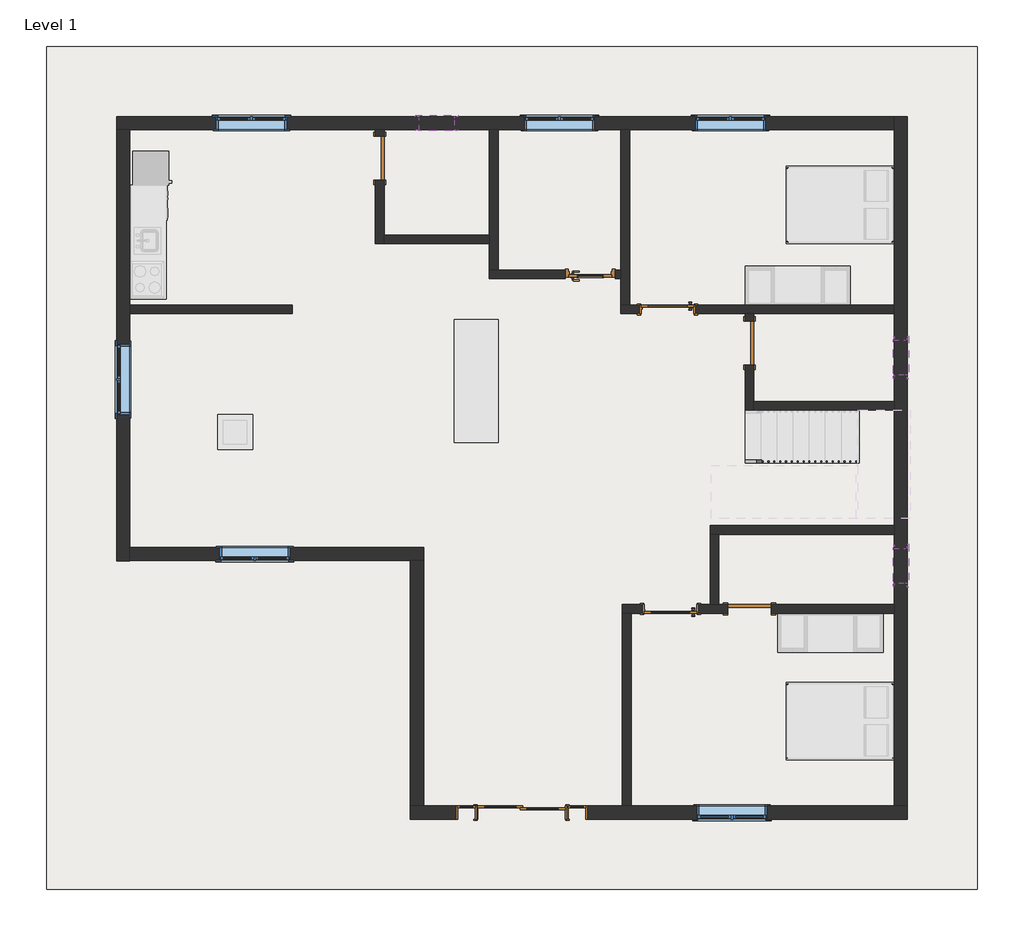
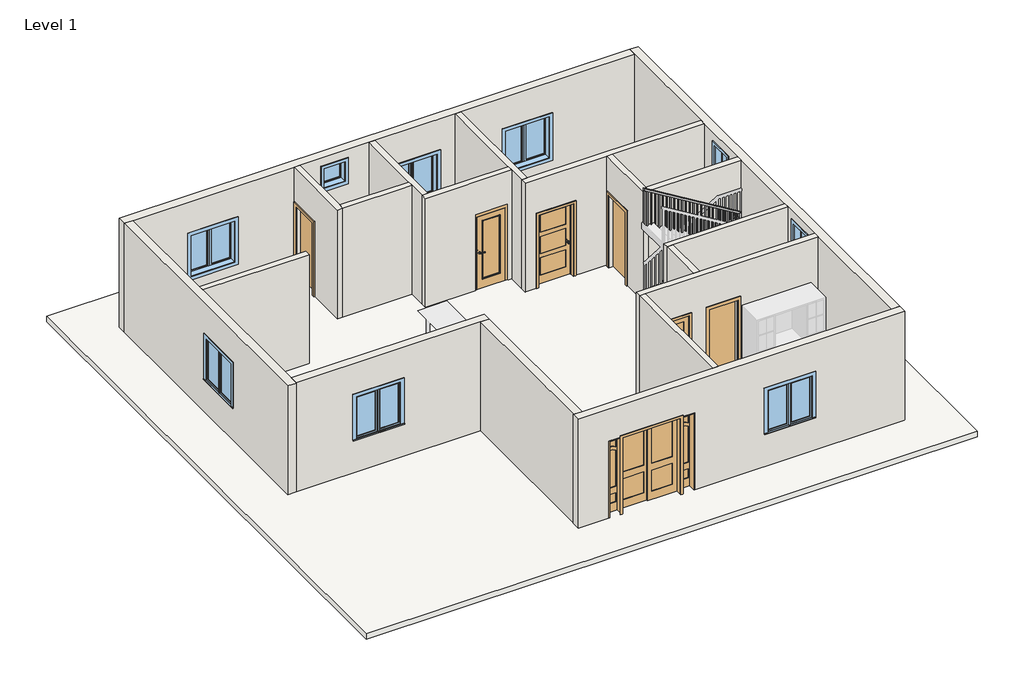
# One storey, part 1 of 2: 19 walls, 9 doors, 9 windows, 1 railing, 1 slab.
"""IFC4 building model written with IfcOpenShell, lengths in millimetres."""

from ifc_helpers import new_model, si_unit, frame, origin, origin_with_axes, place, context, project, spatial, polyline, outline, extrude, faceted_brep, transform, mapped, element, save
from components import door_0052078e, door_302e125b, door_f5864cb8, door_ac27962c, door_c5233792, door_136239c3, door_d64d7266, window_534dcd48, window_3ed046d9

model = new_model("IFC4")

# Units and contexts
model_context = context("Model", 3, world=origin())
ifc_project = project(units=[si_unit("LENGTHUNIT", "METRE", prefix="MILLI")], contexts=[model_context])

# Site, building, storey
site = spatial("IfcSite", under=ifc_project)
building = spatial("IfcBuilding", under=site)
storey = spatial("IfcBuildingStorey", under=building, Name="Level 1", Elevation=0.0)

# Doors
placement = place(None, origin())
door_shape = door_0052078e(model_context)
element("IfcDoor", 1, ObjectType="12\" x 84\"", at=placement, inside=storey, context=model_context, shape_type="MappedRepresentation", body=[
    mapped(door_shape, transform((-8475.4866603, -9530.4581121, 0.0), x_axis=(1.0, 0.0, 0.0), y_axis=(0.0, 1.0, 0.0), z_axis=(0.0, 0.0, 1.0))),
])
door_2_shape = door_302e125b(model_context)
element("IfcDoor", 2, ObjectType="12\" x 84\"", at=placement, inside=storey, context=model_context, shape_type="MappedRepresentation", body=[
    mapped(door_2_shape, transform((-6557.7866603, -9530.4581121, 0.0), x_axis=(-1.0, 0.0, 0.0), y_axis=(0.0, -1.0, 0.0), z_axis=(0.0, 0.0, 1.0))),
])
door_3_shape = door_f5864cb8(model_context)
element("IfcDoor", 3, ObjectType="Door-Interior-Double-Sliding-2_Panel-Wood : 60\" x 84\"", at=placement, inside=storey, context=model_context, shape_type="MappedRepresentation", body=[
    mapped(door_3_shape, transform((-7522.9866603, -9530.4581121, 0.0), x_axis=(1.0, 0.0, 0.0), y_axis=(0.0, 1.0, 0.0), z_axis=(0.0, 0.0, 1.0))),
])
door_4_shape = door_ac27962c(model_context)
element("IfcDoor", 4, ObjectType="Door-Interior-Single-3_Panel_Vert-Wood : 36\" x 80\"", at=placement, inside=storey, context=model_context, shape_type="MappedRepresentation", body=[
    mapped(door_4_shape, transform((-4932.1866603, -5993.5081121, 0.0), x_axis=(-1.0, 0.0, 0.0), y_axis=(0.0, -1.0, 0.0), z_axis=(0.0, 0.0, 1.0))),
])
door_5_shape = door_c5233792(model_context)
element("IfcDoor", 5, ObjectType="Door-Interior-Single-3_Panel_Vert-Wood : 36\" x 80\"", at=placement, inside=storey, context=model_context, shape_type="MappedRepresentation", body=[
    mapped(door_5_shape, transform((-4982.9866603, -780.1581121, 0.0), x_axis=(-1.0, 0.0, 0.0), y_axis=(0.0, -1.0, 0.0), z_axis=(0.0, 0.0, 1.0))),
])
door_6_shape = door_136239c3(model_context)
element("IfcDoor", 6, ObjectType="Door-Passage-Single-Full_Lite : 30\" x 80\"", at=placement, inside=storey, context=model_context, shape_type="MappedRepresentation", body=[
    mapped(door_6_shape, transform((-6329.1866603, -167.3831121, 0.0), x_axis=(1.0, 0.0, 0.0), y_axis=(0.0, 1.0, 0.0), z_axis=(0.0, 0.0, 1.0))),
])
door_7_shape = door_d64d7266(model_context)
element("IfcDoor", 7, ObjectType="Door-Single-Panel : 30\" x 80\"", at=placement, inside=storey, context=model_context, shape_type="MappedRepresentation", body=[
    mapped(door_7_shape, transform((-3560.5866603, -5990.3331121, 0.0), x_axis=(-1.0, 0.0, 0.0), y_axis=(0.0, -1.0, 0.0), z_axis=(0.0, 0.0, 1.0))),
])
element("IfcDoor", 8, ObjectType="Door-Single-Panel : 30\" x 80\"", at=placement, inside=storey, context=model_context, shape_type="MappedRepresentation", body=[
    mapped(door_7_shape, transform((-3560.5866603, -1367.5331121, 0.0), x_axis=(0.0, 1.0, 0.0), y_axis=(-1.0, 0.0, 0.0), z_axis=(0.0, 0.0, 1.0))),
])
element("IfcDoor", 9, ObjectType="Door-Single-Panel : 30\" x 80\"", at=placement, inside=storey, context=model_context, shape_type="MappedRepresentation", body=[
    mapped(door_7_shape, transform((-9986.7866603, 1845.5668879, 0.0), x_axis=(0.0, 1.0, 0.0), y_axis=(-1.0, 0.0, 0.0), z_axis=(0.0, 0.0, 1.0))),
])

# Railing
element("IfcRailing", 10, ObjectType="Handrail - Rectangular", at=placement, inside=storey, context=model_context, shape_type="SolidModel", body=[
    faceted_brep([(-3636.7866603, -3399.5331121, 1083.7333333), (-3636.7866603, -3399.5331121, 1024.3318731), (-3636.7866603, -3450.3331121, 1024.3318731), (-3636.7866603, -3450.3331121, 1083.7333333), (-1757.1866603, -3399.5331121, 2222.8848485), (-1706.3866603, -3399.5331121, 2194.271267), (-1706.3866603, -3450.3331121, 2194.271267), (-1757.1866603, -3450.3331121, 2222.8848485), (-1757.1866603, -3399.5331121, 2269.0666667), (-1706.3866603, -3399.5331121, 2218.2666667), (-1706.3866603, -3450.3331121, 2218.2666667), (-1757.1866603, -3450.3331121, 2269.0666667), (-1630.1866603, -3399.5331121, 2269.0666667), (-1630.1866603, -3399.5331121, 2218.2666667), (-1680.9866603, -3450.3331121, 2218.2666667), (-1680.9866603, -3450.3331121, 2269.0666667), (-1630.1866603, -3501.1331121, 2269.0666667), (-1680.9866603, -3501.1331121, 2269.0666667), (-1680.9866603, -3551.9331121, 2218.2666667), (-1630.1866603, -3551.9331121, 2218.2666667)], [[[0, 1, 2, 3]], [[1, 0, 4, 5]], [[2, 1, 5, 6]], [[3, 2, 6, 7]], [[0, 3, 7, 4]], [[5, 4, 8, 9]], [[6, 5, 9, 10]], [[7, 6, 10, 11]], [[4, 7, 11, 8]], [[9, 8, 12, 13]], [[10, 9, 13, 14]], [[11, 10, 14, 15]], [[8, 11, 15, 12]], [[16, 17, 18, 19]], [[13, 12, 16, 19]], [[14, 13, 19, 18]], [[15, 14, 18, 17]], [[12, 15, 17, 16]]]),
    faceted_brep([(-1630.1866603, -3501.1331121, 2269.0666667), (-1630.1866603, -3551.9331121, 2218.2666667), (-1680.9866603, -3551.9331121, 2218.2666667), (-1680.9866603, -3501.1331121, 2269.0666667), (-1630.1866603, -3501.1331121, 2407.6121212), (-1680.9866603, -3501.1331121, 2378.9985397), (-1680.9866603, -3551.9331121, 2378.9985397), (-1630.1866603, -3551.9331121, 2407.6121212)], [[[0, 1, 2, 3]], [[4, 5, 6, 7]], [[1, 0, 4, 7]], [[2, 1, 7, 6]], [[3, 2, 6, 5]], [[0, 3, 5, 4]]]),
    faceted_brep([(-1630.1866603, -3551.9331121, 2407.6121212), (-1680.9866603, -3551.9331121, 2378.9985397), (-1680.9866603, -3501.1331121, 2378.9985397), (-1630.1866603, -3501.1331121, 2407.6121212), (-4195.5866603, -3551.9331121, 3962.4), (-4195.5866603, -3501.1331121, 3962.4), (-4195.5866603, -3501.1331121, 3902.9985397), (-4195.5866603, -3551.9331121, 3902.9985397)], [[[0, 1, 2, 3]], [[4, 5, 6, 7]], [[1, 0, 4, 7]], [[2, 1, 7, 6]], [[3, 2, 6, 5]], [[0, 3, 5, 4]]]),
    extrude(outline(polyline([(3835.6500549, -4084.4616603), (3847.1955094, -4103.5116603), (2878.6666667, -4103.5116603), (2878.6666667, -4084.4616603), (3835.6500549, -4084.4616603)])), frame((0.0, -3536.0581121, 0.0), z_axis=(0.0, 1.0, 0.0), x_axis=(0.0, 0.0, 1.0)), (0.0, 0.0, 1.0), 19.05),
    extrude(outline(polyline([(3774.0742973, -3982.8616603), (3785.6197519, -4001.9116603), (2878.6666667, -4001.9116603), (2878.6666667, -3982.8616603), (3774.0742973, -3982.8616603)])), frame((0.0, -3536.0581121, 0.0), z_axis=(0.0, 1.0, 0.0), x_axis=(0.0, 0.0, 1.0)), (0.0, 0.0, 1.0), 19.05),
    extrude(outline(polyline([(3712.4985397, -3881.2616603), (3724.0439943, -3900.3116603), (2709.3333333, -3900.3116603), (2709.3333333, -3881.2616603), (3712.4985397, -3881.2616603)])), frame((0.0, -3536.0581121, 0.0), z_axis=(0.0, 1.0, 0.0), x_axis=(0.0, 0.0, 1.0)), (0.0, 0.0, 1.0), 19.05),
    extrude(outline(polyline([(3650.9227822, -3779.6616603), (3662.4682367, -3798.7116603), (2709.3333333, -3798.7116603), (2709.3333333, -3779.6616603), (3650.9227822, -3779.6616603)])), frame((0.0, -3536.0581121, 0.0), z_axis=(0.0, 1.0, 0.0), x_axis=(0.0, 0.0, 1.0)), (0.0, 0.0, 1.0), 19.05),
    extrude(outline(polyline([(3589.3470246, -3678.0616603), (3600.8924791, -3697.1116603), (2709.3333333, -3697.1116603), (2709.3333333, -3678.0616603), (3589.3470246, -3678.0616603)])), frame((0.0, -3536.0581121, 0.0), z_axis=(0.0, 1.0, 0.0), x_axis=(0.0, 0.0, 1.0)), (0.0, 0.0, 1.0), 19.05),
    extrude(outline(polyline([(3527.771267, -3576.4616603), (3539.3167216, -3595.5116603), (2540.0, -3595.5116603), (2540.0, -3576.4616603), (3527.771267, -3576.4616603)])), frame((0.0, -3536.0581121, 0.0), z_axis=(0.0, 1.0, 0.0), x_axis=(0.0, 0.0, 1.0)), (0.0, 0.0, 1.0), 19.05),
    extrude(outline(polyline([(3466.1955094, -3474.8616603), (3477.740964, -3493.9116603), (2540.0, -3493.9116603), (2540.0, -3474.8616603), (3466.1955094, -3474.8616603)])), frame((0.0, -3536.0581121, 0.0), z_axis=(0.0, 1.0, 0.0), x_axis=(0.0, 0.0, 1.0)), (0.0, 0.0, 1.0), 19.05),
    extrude(outline(polyline([(3404.6197519, -3373.2616603), (3416.1652064, -3392.3116603), (2540.0, -3392.3116603), (2540.0, -3373.2616603), (3404.6197519, -3373.2616603)])), frame((0.0, -3536.0581121, 0.0), z_axis=(0.0, 1.0, 0.0), x_axis=(0.0, 0.0, 1.0)), (0.0, 0.0, 1.0), 19.05),
    extrude(outline(polyline([(3343.0439943, -3271.6616603), (3354.5894488, -3290.7116603), (2370.6666667, -3290.7116603), (2370.6666667, -3271.6616603), (3343.0439943, -3271.6616603)])), frame((0.0, -3536.0581121, 0.0), z_axis=(0.0, 1.0, 0.0), x_axis=(0.0, 0.0, 1.0)), (0.0, 0.0, 1.0), 19.05),
    extrude(outline(polyline([(3281.4682367, -3170.0616603), (3293.0136913, -3189.1116603), (2370.6666667, -3189.1116603), (2370.6666667, -3170.0616603), (3281.4682367, -3170.0616603)])), frame((0.0, -3536.0581121, 0.0), z_axis=(0.0, 1.0, 0.0), x_axis=(0.0, 0.0, 1.0)), (0.0, 0.0, 1.0), 19.05),
    extrude(outline(polyline([(3219.8924791, -3068.4616603), (3231.4379337, -3087.5116603), (2370.6666667, -3087.5116603), (2370.6666667, -3068.4616603), (3219.8924791, -3068.4616603)])), frame((0.0, -3536.0581121, 0.0), z_axis=(0.0, 1.0, 0.0), x_axis=(0.0, 0.0, 1.0)), (0.0, 0.0, 1.0), 19.05),
    extrude(outline(polyline([(3158.3167216, -2966.8616603), (3169.8621761, -2985.9116603), (2201.3333333, -2985.9116603), (2201.3333333, -2966.8616603), (3158.3167216, -2966.8616603)])), frame((0.0, -3536.0581121, 0.0), z_axis=(0.0, 1.0, 0.0), x_axis=(0.0, 0.0, 1.0)), (0.0, 0.0, 1.0), 19.05),
    extrude(outline(polyline([(3096.740964, -2865.2616603), (3108.2864185, -2884.3116603), (2201.3333333, -2884.3116603), (2201.3333333, -2865.2616603), (3096.740964, -2865.2616603)])), frame((0.0, -3536.0581121, 0.0), z_axis=(0.0, 1.0, 0.0), x_axis=(0.0, 0.0, 1.0)), (0.0, 0.0, 1.0), 19.05),
    extrude(outline(polyline([(3035.1652064, -2763.6616603), (3046.710661, -2782.7116603), (2032.0, -2782.7116603), (2032.0, -2763.6616603), (3035.1652064, -2763.6616603)])), frame((0.0, -3536.0581121, 0.0), z_axis=(0.0, 1.0, 0.0), x_axis=(0.0, 0.0, 1.0)), (0.0, 0.0, 1.0), 19.05),
    extrude(outline(polyline([(2973.5894488, -2662.0616603), (2985.1349034, -2681.1116603), (2032.0, -2681.1116603), (2032.0, -2662.0616603), (2973.5894488, -2662.0616603)])), frame((0.0, -3536.0581121, 0.0), z_axis=(0.0, 1.0, 0.0), x_axis=(0.0, 0.0, 1.0)), (0.0, 0.0, 1.0), 19.05),
    extrude(outline(polyline([(2912.0136913, -2560.4616603), (2923.5591458, -2579.5116603), (2032.0, -2579.5116603), (2032.0, -2560.4616603), (2912.0136913, -2560.4616603)])), frame((0.0, -3536.0581121, 0.0), z_axis=(0.0, 1.0, 0.0), x_axis=(0.0, 0.0, 1.0)), (0.0, 0.0, 1.0), 19.05),
    extrude(outline(polyline([(2850.4379337, -2458.8616603), (2861.9833882, -2477.9116603), (1862.6666667, -2477.9116603), (1862.6666667, -2458.8616603), (2850.4379337, -2458.8616603)])), frame((0.0, -3536.0581121, 0.0), z_axis=(0.0, 1.0, 0.0), x_axis=(0.0, 0.0, 1.0)), (0.0, 0.0, 1.0), 19.05),
    extrude(outline(polyline([(2788.8621761, -2357.2616603), (2800.4076307, -2376.3116603), (1862.6666667, -2376.3116603), (1862.6666667, -2357.2616603), (2788.8621761, -2357.2616603)])), frame((0.0, -3536.0581121, 0.0), z_axis=(0.0, 1.0, 0.0), x_axis=(0.0, 0.0, 1.0)), (0.0, 0.0, 1.0), 19.05),
    extrude(outline(polyline([(2727.2864185, -2255.6616603), (2738.8318731, -2274.7116603), (1862.6666667, -2274.7116603), (1862.6666667, -2255.6616603), (2727.2864185, -2255.6616603)])), frame((0.0, -3536.0581121, 0.0), z_axis=(0.0, 1.0, 0.0), x_axis=(0.0, 0.0, 1.0)), (0.0, 0.0, 1.0), 19.05),
    extrude(outline(polyline([(2665.710661, -2154.0616603), (2677.2561155, -2173.1116603), (1693.3333333, -2173.1116603), (1693.3333333, -2154.0616603), (2665.710661, -2154.0616603)])), frame((0.0, -3536.0581121, 0.0), z_axis=(0.0, 1.0, 0.0), x_axis=(0.0, 0.0, 1.0)), (0.0, 0.0, 1.0), 19.05),
    extrude(outline(polyline([(2604.1349034, -2052.4616603), (2615.6803579, -2071.5116603), (1693.3333333, -2071.5116603), (1693.3333333, -2052.4616603), (2604.1349034, -2052.4616603)])), frame((0.0, -3536.0581121, 0.0), z_axis=(0.0, 1.0, 0.0), x_axis=(0.0, 0.0, 1.0)), (0.0, 0.0, 1.0), 19.05),
    extrude(outline(polyline([(2542.5591458, -1950.8616603), (2554.1046004, -1969.9116603), (1693.3333333, -1969.9116603), (1693.3333333, -1950.8616603), (2542.5591458, -1950.8616603)])), frame((0.0, -3536.0581121, 0.0), z_axis=(0.0, 1.0, 0.0), x_axis=(0.0, 0.0, 1.0)), (0.0, 0.0, 1.0), 19.05),
    extrude(outline(polyline([(2480.9833882, -1849.2616603), (2492.5288428, -1868.3116603), (1524.0, -1868.3116603), (1524.0, -1849.2616603), (2480.9833882, -1849.2616603)])), frame((0.0, -3536.0581121, 0.0), z_axis=(0.0, 1.0, 0.0), x_axis=(0.0, 0.0, 1.0)), (0.0, 0.0, 1.0), 19.05),
    extrude(outline(polyline([(2419.4076307, -1747.6616603), (2430.9530852, -1766.7116603), (1524.0, -1766.7116603), (1524.0, -1747.6616603), (2419.4076307, -1747.6616603)])), frame((0.0, -3536.0581121, 0.0), z_axis=(0.0, 1.0, 0.0), x_axis=(0.0, 0.0, 1.0)), (0.0, 0.0, 1.0), 19.05),
    extrude(outline(polyline([(2200.0439943, -1696.8616603), (2188.4985397, -1715.9116603), (1185.3333333, -1715.9116603), (1185.3333333, -1696.8616603), (2200.0439943, -1696.8616603)])), frame((0.0, -3434.4581121, 0.0), z_axis=(0.0, 1.0, 0.0), x_axis=(0.0, 0.0, 1.0)), (0.0, 0.0, 1.0), 19.05),
    extrude(outline(polyline([(2138.4682367, -1798.4616603), (2126.9227822, -1817.5116603), (1185.3333333, -1817.5116603), (1185.3333333, -1798.4616603), (2138.4682367, -1798.4616603)])), frame((0.0, -3434.4581121, 0.0), z_axis=(0.0, 1.0, 0.0), x_axis=(0.0, 0.0, 1.0)), (0.0, 0.0, 1.0), 19.05),
    extrude(outline(polyline([(2076.8924791, -1900.0616603), (2065.3470246, -1919.1116603), (1185.3333333, -1919.1116603), (1185.3333333, -1900.0616603), (2076.8924791, -1900.0616603)])), frame((0.0, -3434.4581121, 0.0), z_axis=(0.0, 1.0, 0.0), x_axis=(0.0, 0.0, 1.0)), (0.0, 0.0, 1.0), 19.05),
    extrude(outline(polyline([(2015.3167216, -2001.6616603), (2003.771267, -2020.7116603), (1016.0, -2020.7116603), (1016.0, -2001.6616603), (2015.3167216, -2001.6616603)])), frame((0.0, -3434.4581121, 0.0), z_axis=(0.0, 1.0, 0.0), x_axis=(0.0, 0.0, 1.0)), (0.0, 0.0, 1.0), 19.05),
    extrude(outline(polyline([(1953.740964, -2103.2616603), (1942.1955094, -2122.3116603), (1016.0, -2122.3116603), (1016.0, -2103.2616603), (1953.740964, -2103.2616603)])), frame((0.0, -3434.4581121, 0.0), z_axis=(0.0, 1.0, 0.0), x_axis=(0.0, 0.0, 1.0)), (0.0, 0.0, 1.0), 19.05),
    extrude(outline(polyline([(1892.1652064, -2204.8616603), (1880.6197519, -2223.9116603), (1016.0, -2223.9116603), (1016.0, -2204.8616603), (1892.1652064, -2204.8616603)])), frame((0.0, -3434.4581121, 0.0), z_axis=(0.0, 1.0, 0.0), x_axis=(0.0, 0.0, 1.0)), (0.0, 0.0, 1.0), 19.05),
    extrude(outline(polyline([(1830.5894488, -2306.4616603), (1819.0439943, -2325.5116603), (846.6666667, -2325.5116603), (846.6666667, -2306.4616603), (1830.5894488, -2306.4616603)])), frame((0.0, -3434.4581121, 0.0), z_axis=(0.0, 1.0, 0.0), x_axis=(0.0, 0.0, 1.0)), (0.0, 0.0, 1.0), 19.05),
    extrude(outline(polyline([(1769.0136913, -2408.0616603), (1757.4682367, -2427.1116603), (846.6666667, -2427.1116603), (846.6666667, -2408.0616603), (1769.0136913, -2408.0616603)])), frame((0.0, -3434.4581121, 0.0), z_axis=(0.0, 1.0, 0.0), x_axis=(0.0, 0.0, 1.0)), (0.0, 0.0, 1.0), 19.05),
    extrude(outline(polyline([(1707.4379337, -2509.6616603), (1695.8924791, -2528.7116603), (846.6666667, -2528.7116603), (846.6666667, -2509.6616603), (1707.4379337, -2509.6616603)])), frame((0.0, -3434.4581121, 0.0), z_axis=(0.0, 1.0, 0.0), x_axis=(0.0, 0.0, 1.0)), (0.0, 0.0, 1.0), 19.05),
    extrude(outline(polyline([(1645.8621761, -2611.2616603), (1634.3167216, -2630.3116603), (677.3333333, -2630.3116603), (677.3333333, -2611.2616603), (1645.8621761, -2611.2616603)])), frame((0.0, -3434.4581121, 0.0), z_axis=(0.0, 1.0, 0.0), x_axis=(0.0, 0.0, 1.0)), (0.0, 0.0, 1.0), 19.05),
    extrude(outline(polyline([(1584.2864185, -2712.8616603), (1572.740964, -2731.9116603), (677.3333333, -2731.9116603), (677.3333333, -2712.8616603), (1584.2864185, -2712.8616603)])), frame((0.0, -3434.4581121, 0.0), z_axis=(0.0, 1.0, 0.0), x_axis=(0.0, 0.0, 1.0)), (0.0, 0.0, 1.0), 19.05),
    extrude(outline(polyline([(1522.710661, -2814.4616603), (1511.1652064, -2833.5116603), (508.0, -2833.5116603), (508.0, -2814.4616603), (1522.710661, -2814.4616603)])), frame((0.0, -3434.4581121, 0.0), z_axis=(0.0, 1.0, 0.0), x_axis=(0.0, 0.0, 1.0)), (0.0, 0.0, 1.0), 19.05),
    extrude(outline(polyline([(1461.1349034, -2916.0616603), (1449.5894488, -2935.1116603), (508.0, -2935.1116603), (508.0, -2916.0616603), (1461.1349034, -2916.0616603)])), frame((0.0, -3434.4581121, 0.0), z_axis=(0.0, 1.0, 0.0), x_axis=(0.0, 0.0, 1.0)), (0.0, 0.0, 1.0), 19.05),
    extrude(outline(polyline([(1399.5591458, -3017.6616603), (1388.0136913, -3036.7116603), (508.0, -3036.7116603), (508.0, -3017.6616603), (1399.5591458, -3017.6616603)])), frame((0.0, -3434.4581121, 0.0), z_axis=(0.0, 1.0, 0.0), x_axis=(0.0, 0.0, 1.0)), (0.0, 0.0, 1.0), 19.05),
    extrude(outline(polyline([(1337.9833882, -3119.2616603), (1326.4379337, -3138.3116603), (338.6666667, -3138.3116603), (338.6666667, -3119.2616603), (1337.9833882, -3119.2616603)])), frame((0.0, -3434.4581121, 0.0), z_axis=(0.0, 1.0, 0.0), x_axis=(0.0, 0.0, 1.0)), (0.0, 0.0, 1.0), 19.05),
    extrude(outline(polyline([(1276.4076307, -3220.8616603), (1264.8621761, -3239.9116603), (338.6666667, -3239.9116603), (338.6666667, -3220.8616603), (1276.4076307, -3220.8616603)])), frame((0.0, -3434.4581121, 0.0), z_axis=(0.0, 1.0, 0.0), x_axis=(0.0, 0.0, 1.0)), (0.0, 0.0, 1.0), 19.05),
    extrude(outline(polyline([(1214.8318731, -3322.4616603), (1203.2864185, -3341.5116603), (338.6666667, -3341.5116603), (338.6666667, -3322.4616603), (1214.8318731, -3322.4616603)])), frame((0.0, -3434.4581121, 0.0), z_axis=(0.0, 1.0, 0.0), x_axis=(0.0, 0.0, 1.0)), (0.0, 0.0, 1.0), 19.05),
    extrude(outline(polyline([(1153.2561155, -3424.0616603), (1141.710661, -3443.1116603), (169.3333333, -3443.1116603), (169.3333333, -3424.0616603), (1153.2561155, -3424.0616603)])), frame((0.0, -3434.4581121, 0.0), z_axis=(0.0, 1.0, 0.0), x_axis=(0.0, 0.0, 1.0)), (0.0, 0.0, 1.0), 19.05),
    extrude(outline(polyline([(1091.6803579, -3525.6616603), (1080.1349034, -3544.7116603), (169.3333333, -3544.7116603), (169.3333333, -3525.6616603), (1091.6803579, -3525.6616603)])), frame((0.0, -3434.4581121, 0.0), z_axis=(0.0, 1.0, 0.0), x_axis=(0.0, 0.0, 1.0)), (0.0, 0.0, 1.0), 19.05),
    extrude(outline(polyline([(-1646.0616603, -3517.0081121), (-1646.0616603, -3536.0581121), (-1665.1116603, -3536.0581121), (-1665.1116603, -3517.0081121), (-1646.0616603, -3517.0081121)])), frame((0.0, 0.0, 1354.6666667), z_axis=(0.0, 0.0, 1.0), x_axis=(1.0, 0.0, 0.0)), (0.0, 0.0, 1.0), 863.6),
    extrude(outline(polyline([(-1665.1116603, -3434.4581121), (-1665.1116603, -3415.4081121), (-1646.0616603, -3415.4081121), (-1646.0616603, -3434.4581121), (-1665.1116603, -3434.4581121)])), frame((0.0, 0.0, 1354.6666667), z_axis=(0.0, 0.0, 1.0), x_axis=(1.0, 0.0, 0.0)), (0.0, 0.0, 1.0), 863.6),
    extrude(outline(polyline([(-1690.5116603, -3434.4581121), (-1690.5116603, -3415.4081121), (-1671.4616603, -3415.4081121), (-1671.4616603, -3434.4581121), (-1690.5116603, -3434.4581121)])), frame((0.0, 0.0, 1354.6666667), z_axis=(0.0, 0.0, 1.0), x_axis=(1.0, 0.0, 0.0)), (0.0, 0.0, 1.0), 863.6),
    extrude(outline(polyline([(3891.4530852, -4176.5366603), (3902.9985397, -4195.5866603), (2878.6666667, -4195.5866603), (2878.6666667, -4176.5366603), (3891.4530852, -4176.5366603)])), frame((0.0, -3536.0581121, 0.0), z_axis=(0.0, 1.0, 0.0), x_axis=(0.0, 0.0, 1.0)), (0.0, 0.0, 1.0), 19.05),
    extrude(outline(polyline([(1035.8773276, -3617.7366603), (1024.3318731, -3636.7866603), (169.3333333, -3636.7866603), (169.3333333, -3617.7366603), (1035.8773276, -3617.7366603)])), frame((0.0, -3434.4581121, 0.0), z_axis=(0.0, 1.0, 0.0), x_axis=(0.0, 0.0, 1.0)), (0.0, 0.0, 1.0), 19.05),
])

# Slab
element("IfcSlab", 11, ObjectType="Generic - 6\" 2", at=placement, inside=storey, context=model_context, shape_type="SweptSolid", body=[
    extrude(outline(polyline([(401.8133397, 3788.6668879), (401.8133397, -10867.1331121), (-15777.9866603, -10867.1331121), (-15777.9866603, 3788.6668879), (401.8133397, 3788.6668879)])), frame((0.0, 0.0, -152.4), z_axis=(0.0, 0.0, 1.0), x_axis=(1.0, 0.0, 0.0)), (0.0, 0.0, 1.0), 152.4),
])

# Walls
element("IfcWall", 12, ObjectType="Generic - 6\"", at=placement, inside=storey, context=model_context, shape_type="SweptSolid", body=[
    extrude(outline(polyline([(-11510.7866603, -859.5331121), (-14330.1866603, -859.5331121), (-14330.1866603, -707.1331121), (-11510.7866603, -707.1331121), (-11510.7866603, -859.5331121)])), origin_with_axes(), (0.0, 0.0, 1.0), 3048.0),
])
element("IfcWall", 13, ObjectType="Generic - 6\"", at=placement, inside=storey, context=model_context, shape_type="Brep", body=[
    faceted_brep([(-10062.9866603, 2340.8668879, 0.0), (-10062.9866603, 2226.5668879, 0.0), (-10062.9866603, 2226.5668879, 2032.0), (-10062.9866603, 1464.5668879, 2032.0), (-10062.9866603, 1464.5668879, 0.0), (-10062.9866603, 359.6668879, 0.0), (-10062.9866603, 359.6668879, 3048.0), (-10062.9866603, 2340.8668879, 3048.0), (-9910.5866603, 2226.5668879, 2032.0), (-9910.5866603, 2226.5668879, 0.0), (-9910.5866603, 2340.8668879, 0.0), (-9910.5866603, 2340.8668879, 3048.0), (-9910.5866603, 512.0668879, 3048.0), (-9910.5866603, 359.6668879, 3048.0), (-9910.5866603, 359.6668879, 0.0), (-9910.5866603, 512.0668879, 0.0), (-9910.5866603, 1464.5668879, 0.0), (-9910.5866603, 1464.5668879, 2032.0)], [[[0, 1, 2, 3, 4, 5, 6, 7]], [[8, 9, 10, 11, 12, 13, 14, 15, 16, 17]], [[10, 9, 1, 0]], [[16, 15, 14, 5, 4]], [[6, 5, 14, 13]], [[7, 6, 13, 12, 11]], [[0, 7, 11, 10]], [[2, 1, 9, 8]], [[3, 2, 8, 17]], [[4, 3, 17, 16]]]),
])
element("IfcWall", 14, ObjectType="Generic - 6\"", at=placement, inside=storey, context=model_context, shape_type="Brep", body=[
    faceted_brep([(-5795.7866603, -707.1331121, 3048.0), (-5643.3866603, -707.1331121, 3048.0), (-1045.9866603, -707.1331121, 3048.0), (-1045.9866603, -707.1331121, 0.0), (-4500.3866603, -707.1331121, 0.0), (-4500.3866603, -707.1331121, 2057.4), (-5465.5866603, -707.1331121, 2057.4), (-5465.5866603, -707.1331121, 0.0), (-5643.3866603, -707.1331121, 0.0), (-5795.7866603, -707.1331121, 0.0), (-1045.9866603, -859.5331121, 3048.0), (-3484.3866603, -859.5331121, 3048.0), (-3636.7866603, -859.5331121, 3048.0), (-5795.7866603, -859.5331121, 3048.0), (-5795.7866603, -859.5331121, 0.0), (-5465.5866603, -859.5331121, 0.0), (-5465.5866603, -859.5331121, 2057.4), (-4500.3866603, -859.5331121, 2057.4), (-4500.3866603, -859.5331121, 0.0), (-3636.7866603, -859.5331121, 0.0), (-3484.3866603, -859.5331121, 0.0), (-1045.9866603, -859.5331121, 0.0)], [[[0, 1, 2, 3, 4, 5, 6, 7, 8, 9]], [[10, 11, 12, 13, 14, 15, 16, 17, 18, 19, 20, 21]], [[3, 21, 20, 19, 18, 4]], [[14, 9, 8, 7, 15]], [[2, 1, 0, 13, 12, 11, 10]], [[3, 2, 10, 21]], [[0, 9, 14, 13]], [[6, 16, 15, 7]], [[16, 6, 5, 17]], [[17, 5, 4, 18]]]),
])
element("IfcWall", 15, ObjectType="Generic - 6\"", at=placement, inside=storey, context=model_context, shape_type="Brep", body=[
    faceted_brep([(-5643.3866603, -707.1331121, 0.0), (-5643.3866603, 2340.8668879, 0.0), (-5643.3866603, 2340.8668879, 3048.0), (-5643.3866603, -707.1331121, 3048.0), (-5795.7866603, -707.1331121, 0.0), (-5795.7866603, -707.1331121, 3048.0), (-5795.7866603, -249.9331121, 3048.0), (-5795.7866603, -97.5331121, 3048.0), (-5795.7866603, 2340.8668879, 3048.0), (-5795.7866603, 2340.8668879, 0.0), (-5795.7866603, -97.5331121, 0.0), (-5795.7866603, -249.9331121, 0.0)], [[[0, 1, 2, 3]], [[4, 5, 6, 7, 8, 9, 10, 11]], [[1, 0, 4, 11, 10, 9]], [[3, 2, 8, 7, 6, 5]], [[0, 3, 5, 4]], [[2, 1, 9, 8]]]),
])
element("IfcWall", 16, ObjectType="Generic - 6\"", at=placement, inside=storey, context=model_context, shape_type="SweptSolid", body=[
    extrude(outline(polyline([(-8081.7866603, 359.6668879), (-9910.5866603, 359.6668879), (-9910.5866603, 512.0668879), (-8081.7866603, 512.0668879), (-8081.7866603, 359.6668879)])), origin_with_axes(), (0.0, 0.0, 1.0), 3048.0),
])
element("IfcWall", 17, ObjectType="Generic - 6\"", at=placement, inside=storey, context=model_context, shape_type="Brep", body=[
    faceted_brep([(-7929.3866603, -97.5331121, 0.0), (-7929.3866603, 2340.8668879, 0.0), (-7929.3866603, 2340.8668879, 3048.0), (-7929.3866603, -97.5331121, 3048.0), (-8081.7866603, -97.5331121, 0.0), (-8081.7866603, -97.5331121, 3048.0), (-8081.7866603, 359.6668879, 3048.0), (-8081.7866603, 512.0668879, 3048.0), (-8081.7866603, 2340.8668879, 3048.0), (-8081.7866603, 2340.8668879, 0.0), (-8081.7866603, 512.0668879, 0.0), (-8081.7866603, 359.6668879, 0.0)], [[[0, 1, 2, 3]], [[4, 5, 6, 7, 8, 9, 10, 11]], [[1, 0, 4, 11, 10, 9]], [[3, 2, 8, 7, 6, 5]], [[2, 1, 9, 8]], [[0, 3, 5, 4]]]),
])
element("IfcWall", 18, ObjectType="Generic - 6\"", at=placement, inside=storey, context=model_context, shape_type="Brep", body=[
    faceted_brep([(-8081.7866603, -97.5331121, 3048.0), (-7929.3866603, -97.5331121, 3048.0), (-5795.7866603, -97.5331121, 3048.0), (-5795.7866603, -97.5331121, 0.0), (-5897.3866603, -97.5331121, 0.0), (-5897.3866603, -97.5331121, 2133.6), (-6760.9866603, -97.5331121, 2133.6), (-6760.9866603, -97.5331121, 0.0), (-7929.3866603, -97.5331121, 0.0), (-8081.7866603, -97.5331121, 0.0), (-5795.7866603, -249.9331121, 3048.0), (-8081.7866603, -249.9331121, 3048.0), (-8081.7866603, -249.9331121, 0.0), (-6760.9866603, -249.9331121, 0.0), (-6760.9866603, -249.9331121, 2133.6), (-5897.3866603, -249.9331121, 2133.6), (-5897.3866603, -249.9331121, 0.0), (-5795.7866603, -249.9331121, 0.0)], [[[0, 1, 2, 3, 4, 5, 6, 7, 8, 9]], [[10, 11, 12, 13, 14, 15, 16, 17]], [[3, 2, 10, 17]], [[0, 9, 12, 11]], [[12, 9, 8, 7, 13]], [[3, 17, 16, 4]], [[2, 1, 0, 11, 10]], [[15, 5, 4, 16]], [[5, 15, 14, 6]], [[6, 14, 13, 7]]]),
])
element("IfcWall", 19, ObjectType="Generic - 6\"", at=placement, inside=storey, context=model_context, shape_type="Brep", body=[
    faceted_brep([(-3636.7866603, -859.5331121, 0.0), (-3636.7866603, -986.5331121, 0.0), (-3636.7866603, -986.5331121, 2032.0), (-3636.7866603, -1748.5331121, 2032.0), (-3636.7866603, -1748.5331121, 0.0), (-3636.7866603, -2535.9331121, 0.0), (-3636.7866603, -2535.9331121, 3048.0), (-3636.7866603, -859.5331121, 3048.0), (-3484.3866603, -986.5331121, 2032.0), (-3484.3866603, -986.5331121, 0.0), (-3484.3866603, -859.5331121, 0.0), (-3484.3866603, -859.5331121, 3048.0), (-3484.3866603, -2383.5331121, 3048.0), (-3484.3866603, -2535.9331121, 3048.0), (-3484.3866603, -2535.9331121, 0.0), (-3484.3866603, -2383.5331121, 0.0), (-3484.3866603, -1748.5331121, 0.0), (-3484.3866603, -1748.5331121, 2032.0)], [[[0, 1, 2, 3, 4, 5, 6, 7]], [[8, 9, 10, 11, 12, 13, 14, 15, 16, 17]], [[10, 9, 1, 0]], [[16, 15, 14, 5, 4]], [[7, 6, 13, 12, 11]], [[0, 7, 11, 10]], [[6, 5, 14, 13]], [[2, 1, 9, 8]], [[3, 2, 8, 17]], [[4, 3, 17, 16]]]),
])
element("IfcWall", 20, ObjectType="Generic - 6\"", at=placement, inside=storey, context=model_context, shape_type="SweptSolid", body=[
    extrude(outline(polyline([(-1045.9866603, -2535.9331121), (-3484.3866603, -2535.9331121), (-3484.3866603, -2383.5331121), (-1045.9866603, -2383.5331121), (-1045.9866603, -2535.9331121)])), origin_with_axes(), (0.0, 0.0, 1.0), 3048.0),
])
element("IfcWall", 21, ObjectType="Generic - 6\"", at=placement, inside=storey, context=model_context, shape_type="Brep", body=[
    faceted_brep([(-3941.5866603, -5914.1331121, 2032.0), (-3941.5866603, -5914.1331121, 0.0), (-4093.9866603, -5914.1331121, 0.0), (-4246.3866603, -5914.1331121, 0.0), (-4449.5866603, -5914.1331121, 0.0), (-4449.5866603, -5914.1331121, 2057.4), (-5414.7866603, -5914.1331121, 2057.4), (-5414.7866603, -5914.1331121, 0.0), (-5770.3866603, -5914.1331121, 0.0), (-5770.3866603, -5914.1331121, 3048.0), (-4246.3866603, -5914.1331121, 3048.0), (-4093.9866603, -5914.1331121, 3048.0), (-1045.9866603, -5914.1331121, 3048.0), (-1045.9866603, -5914.1331121, 0.0), (-3179.5866603, -5914.1331121, 0.0), (-3179.5866603, -5914.1331121, 2032.0), (-4449.5866603, -6066.5331121, 0.0), (-3941.5866603, -6066.5331121, 0.0), (-3941.5866603, -6066.5331121, 2032.0), (-3179.5866603, -6066.5331121, 2032.0), (-3179.5866603, -6066.5331121, 0.0), (-1045.9866603, -6066.5331121, 0.0), (-1045.9866603, -6066.5331121, 3048.0), (-5617.9866603, -6066.5331121, 3048.0), (-5770.3866603, -6066.5331121, 3048.0), (-5770.3866603, -6066.5331121, 0.0), (-5617.9866603, -6066.5331121, 0.0), (-5414.7866603, -6066.5331121, 0.0), (-5414.7866603, -6066.5331121, 2057.4), (-4449.5866603, -6066.5331121, 2057.4)], [[[0, 1, 2, 3, 4, 5, 6, 7, 8, 9, 10, 11, 12, 13, 14, 15]], [[16, 17, 18, 19, 20, 21, 22, 23, 24, 25, 26, 27, 28, 29]], [[25, 8, 7, 27, 26]], [[14, 13, 21, 20]], [[4, 3, 2, 1, 17, 16]], [[12, 11, 10, 9, 24, 23, 22]], [[13, 12, 22, 21]], [[9, 8, 25, 24]], [[6, 28, 27, 7]], [[28, 6, 5, 29]], [[29, 5, 4, 16]], [[18, 17, 1, 0]], [[19, 18, 0, 15]], [[20, 19, 15, 14]]]),
])
element("IfcWall", 22, ObjectType="Generic - 6\"", at=placement, inside=storey, context=model_context, shape_type="SweptSolid", body=[
    extrude(outline(polyline([(-5770.3866603, -9419.3331121), (-5770.3866603, -6066.5331121), (-5617.9866603, -6066.5331121), (-5617.9866603, -9419.3331121), (-5770.3866603, -9419.3331121)])), origin_with_axes(), (0.0, 0.0, 1.0), 3048.0),
])
element("IfcWall", 23, ObjectType="Generic - 6\"", at=placement, inside=storey, context=model_context, shape_type="Brep", body=[
    faceted_brep([(-1045.9866603, -4542.5331121, 0.0), (-4246.3866603, -4542.5331121, 0.0), (-4246.3866603, -4542.5331121, 3048.0), (-1045.9866603, -4542.5331121, 3048.0), (-1045.9866603, -4694.9331121, 0.0), (-1045.9866603, -4694.9331121, 3048.0), (-4093.9866603, -4694.9331121, 3048.0), (-4246.3866603, -4694.9331121, 3048.0), (-4246.3866603, -4694.9331121, 0.0), (-4093.9866603, -4694.9331121, 0.0)], [[[0, 1, 2, 3]], [[4, 5, 6, 7, 8, 9]], [[1, 0, 4, 9, 8]], [[3, 2, 7, 6, 5]], [[0, 3, 5, 4]], [[2, 1, 8, 7]]]),
])
element("IfcWall", 24, ObjectType="Generic - 6\"", at=placement, inside=storey, context=model_context, shape_type="SweptSolid", body=[
    extrude(outline(polyline([(-4246.3866603, -5914.1331121), (-4246.3866603, -4694.9331121), (-4093.9866603, -4694.9331121), (-4093.9866603, -5914.1331121), (-4246.3866603, -5914.1331121)])), origin_with_axes(), (0.0, 0.0, 1.0), 3048.0),
])
element("IfcWall", 25, ObjectType="Generic - 9\" 2", at=placement, inside=storey, context=model_context, shape_type="Brep", body=[
    faceted_brep([(-14558.7866603, 2340.8668879, 0.0), (-14330.1866603, 2340.8668879, 0.0), (-10062.9866603, 2340.8668879, 0.0), (-9910.5866603, 2340.8668879, 0.0), (-8081.7866603, 2340.8668879, 0.0), (-7929.3866603, 2340.8668879, 0.0), (-5795.7866603, 2340.8668879, 0.0), (-5643.3866603, 2340.8668879, 0.0), (-1045.9866603, 2340.8668879, 0.0), (-1045.9866603, 2340.8668879, 3048.0), (-5643.3866603, 2340.8668879, 3048.0), (-5795.7866603, 2340.8668879, 3048.0), (-7929.3866603, 2340.8668879, 3048.0), (-8081.7866603, 2340.8668879, 3048.0), (-9910.5866603, 2340.8668879, 3048.0), (-10062.9866603, 2340.8668879, 3048.0), (-14330.1866603, 2340.8668879, 3048.0), (-14558.7866603, 2340.8668879, 3048.0), (-11606.0366603, 2340.8668879, 2133.6), (-11606.0366603, 2340.8668879, 914.4), (-12825.2366603, 2340.8668879, 914.4), (-12825.2366603, 2340.8668879, 2133.6), (-6252.9866603, 2340.8668879, 2133.6), (-6252.9866603, 2340.8668879, 914.4), (-7472.1866603, 2340.8668879, 914.4), (-7472.1866603, 2340.8668879, 2133.6), (-3281.1866603, 2340.8668879, 2133.6), (-3281.1866603, 2340.8668879, 914.4), (-4500.3866603, 2340.8668879, 914.4), (-4500.3866603, 2340.8668879, 2133.6), (-8691.3866603, 2340.8668879, 2768.6), (-8691.3866603, 2340.8668879, 2159.0), (-9300.9866603, 2340.8668879, 2159.0), (-9300.9866603, 2340.8668879, 2768.6), (-14558.7866603, 2569.4668879, 0.0), (-14558.7866603, 2569.4668879, 3048.0), (-1045.9866603, 2569.4668879, 3048.0), (-1045.9866603, 2569.4668879, 0.0), (-11606.0366603, 2569.4668879, 2133.6), (-12825.2366603, 2569.4668879, 2133.6), (-12825.2366603, 2569.4668879, 914.4), (-11606.0366603, 2569.4668879, 914.4), (-6252.9866603, 2569.4668879, 2133.6), (-7472.1866603, 2569.4668879, 2133.6), (-7472.1866603, 2569.4668879, 914.4), (-6252.9866603, 2569.4668879, 914.4), (-3281.1866603, 2569.4668879, 2133.6), (-4500.3866603, 2569.4668879, 2133.6), (-4500.3866603, 2569.4668879, 914.4), (-3281.1866603, 2569.4668879, 914.4), (-8691.3866603, 2569.4668879, 2768.6), (-9300.9866603, 2569.4668879, 2768.6), (-9300.9866603, 2569.4668879, 2159.0), (-8691.3866603, 2569.4668879, 2159.0)], [[[0, 1, 2, 3, 4, 5, 6, 7, 8, 9, 10, 11, 12, 13, 14, 15, 16, 17], [18, 19, 20, 21], [22, 23, 24, 25], [26, 27, 28, 29], [30, 31, 32, 33]], [[34, 35, 36, 37], [38, 39, 40, 41], [42, 43, 44, 45], [46, 47, 48, 49], [50, 51, 52, 53]], [[8, 7, 6, 5, 4, 3, 2, 1, 0, 34, 37]], [[17, 16, 15, 14, 13, 12, 11, 10, 9, 36, 35]], [[0, 17, 35, 34]], [[9, 8, 37, 36]], [[19, 18, 38, 41]], [[20, 19, 41, 40]], [[21, 20, 40, 39]], [[18, 21, 39, 38]], [[23, 22, 42, 45]], [[24, 23, 45, 44]], [[25, 24, 44, 43]], [[22, 25, 43, 42]], [[27, 26, 46, 49]], [[28, 27, 49, 48]], [[29, 28, 48, 47]], [[26, 29, 47, 46]], [[31, 30, 50, 53]], [[32, 31, 53, 52]], [[33, 32, 52, 51]], [[30, 33, 51, 50]]]),
])
element("IfcWall", 26, ObjectType="Generic - 9\" 2", at=placement, inside=storey, context=model_context, shape_type="Brep", body=[
    faceted_brep([(-9459.7366603, -9419.3331121, 0.0), (-9459.7366603, -9419.3331121, 3048.0), (-9453.3866603, -9419.3331121, 3048.0), (-9224.7866603, -9419.3331121, 3048.0), (-5770.3866603, -9419.3331121, 3048.0), (-5617.9866603, -9419.3331121, 3048.0), (-1045.9866603, -9419.3331121, 3048.0), (-817.3866603, -9419.3331121, 3048.0), (-817.3866603, -9419.3331121, 0.0), (-1045.9866603, -9419.3331121, 0.0), (-5617.9866603, -9419.3331121, 0.0), (-5770.3866603, -9419.3331121, 0.0), (-6379.9866603, -9419.3331121, 0.0), (-6379.9866603, -9419.3331121, 2159.0), (-8653.2866603, -9419.3331121, 2159.0), (-8653.2866603, -9419.3331121, 0.0), (-9224.7866603, -9419.3331121, 0.0), (-9453.3866603, -9419.3331121, 0.0), (-4474.9866603, -9419.3331121, 2133.6), (-4474.9866603, -9419.3331121, 914.4), (-3255.7866603, -9419.3331121, 914.4), (-3255.7866603, -9419.3331121, 2133.6), (-9459.7366603, -9647.9331121, 3048.0), (-9459.7366603, -9647.9331121, 0.0), (-8653.2866603, -9647.9331121, 0.0), (-8653.2866603, -9647.9331121, 2159.0), (-6379.9866603, -9647.9331121, 2159.0), (-6379.9866603, -9647.9331121, 0.0), (-817.3866603, -9647.9331121, 0.0), (-817.3866603, -9647.9331121, 3048.0), (-4474.9866603, -9647.9331121, 914.4), (-4474.9866603, -9647.9331121, 2133.6), (-3255.7866603, -9647.9331121, 2133.6), (-3255.7866603, -9647.9331121, 914.4)], [[[0, 1, 2, 3, 4, 5, 6, 7, 8, 9, 10, 11, 12, 13, 14, 15, 16, 17], [18, 19, 20, 21]], [[22, 23, 24, 25, 26, 27, 28, 29], [30, 31, 32, 33]], [[23, 0, 17, 16, 15, 24]], [[8, 28, 27, 12, 11, 10, 9]], [[1, 0, 23, 22]], [[7, 6, 5, 4, 3, 2, 1, 22, 29]], [[8, 7, 29, 28]], [[19, 18, 31, 30]], [[20, 19, 30, 33]], [[21, 20, 33, 32]], [[18, 21, 32, 31]], [[25, 14, 13, 26]], [[14, 25, 24, 15]], [[26, 13, 12, 27]]]),
])
element("IfcWall", 27, ObjectType="Generic - 9\" 2", at=placement, inside=storey, context=model_context, shape_type="Brep", body=[
    faceted_brep([(-1045.9866603, 2569.4668879, 0.0), (-1045.9866603, 2340.8668879, 0.0), (-1045.9866603, -707.1331121, 0.0), (-1045.9866603, -859.5331121, 0.0), (-1045.9866603, -2383.5331121, 0.0), (-1045.9866603, -2535.9331121, 0.0), (-1045.9866603, -4542.5331121, 0.0), (-1045.9866603, -4694.9331121, 0.0), (-1045.9866603, -5914.1331121, 0.0), (-1045.9866603, -6066.5331121, 0.0), (-1045.9866603, -9419.3331121, 0.0), (-1045.9866603, -9419.3331121, 3048.0), (-1045.9866603, -6066.5331121, 3048.0), (-1045.9866603, -5914.1331121, 3048.0), (-1045.9866603, -4694.9331121, 3048.0), (-1045.9866603, -4542.5331121, 3048.0), (-1045.9866603, -2535.9331121, 3048.0), (-1045.9866603, -2383.5331121, 3048.0), (-1045.9866603, -859.5331121, 3048.0), (-1045.9866603, -707.1331121, 3048.0), (-1045.9866603, 2340.8668879, 3048.0), (-1045.9866603, 2569.4668879, 3048.0), (-1045.9866603, -5545.8331121, 2768.6), (-1045.9866603, -5545.8331121, 2159.0), (-1045.9866603, -4936.2331121, 2159.0), (-1045.9866603, -4936.2331121, 2768.6), (-1045.9866603, -1926.3331121, 2768.6), (-1045.9866603, -1926.3331121, 2159.0), (-1045.9866603, -1316.7331121, 2159.0), (-1045.9866603, -1316.7331121, 2768.6), (-817.3866603, 2569.4668879, 0.0), (-817.3866603, 2569.4668879, 3048.0), (-817.3866603, -9419.3331121, 3048.0), (-817.3866603, -9419.3331121, 0.0), (-817.3866603, -5545.8331121, 2768.6), (-817.3866603, -4936.2331121, 2768.6), (-817.3866603, -4936.2331121, 2159.0), (-817.3866603, -5545.8331121, 2159.0), (-817.3866603, -1926.3331121, 2768.6), (-817.3866603, -1316.7331121, 2768.6), (-817.3866603, -1316.7331121, 2159.0), (-817.3866603, -1926.3331121, 2159.0)], [[[0, 1, 2, 3, 4, 5, 6, 7, 8, 9, 10, 11, 12, 13, 14, 15, 16, 17, 18, 19, 20, 21], [22, 23, 24, 25], [26, 27, 28, 29]], [[30, 31, 32, 33], [34, 35, 36, 37], [38, 39, 40, 41]], [[10, 9, 8, 7, 6, 5, 4, 3, 2, 1, 0, 30, 33]], [[21, 20, 19, 18, 17, 16, 15, 14, 13, 12, 11, 32, 31]], [[0, 21, 31, 30]], [[11, 10, 33, 32]], [[23, 22, 34, 37]], [[24, 23, 37, 36]], [[25, 24, 36, 35]], [[22, 25, 35, 34]], [[27, 26, 38, 41]], [[28, 27, 41, 40]], [[29, 28, 40, 39]], [[26, 29, 39, 38]]]),
])
element("IfcWall", 28, ObjectType="Generic - 9\" 2", at=placement, inside=storey, context=model_context, shape_type="Brep", body=[
    faceted_brep([(-14330.1866603, -5152.1331121, 0.0), (-9453.3866603, -5152.1331121, 0.0), (-9224.7866603, -5152.1331121, 0.0), (-9224.7866603, -5152.1331121, 3048.0), (-9453.3866603, -5152.1331121, 3048.0), (-14330.1866603, -5152.1331121, 3048.0), (-12768.0866603, -5152.1331121, 2133.6), (-11548.8866603, -5152.1331121, 2133.6), (-11548.8866603, -5152.1331121, 914.4), (-12768.0866603, -5152.1331121, 914.4), (-14330.1866603, -4923.5331121, 0.0), (-14330.1866603, -4923.5331121, 3048.0), (-9224.7866603, -4923.5331121, 3048.0), (-9224.7866603, -4923.5331121, 0.0), (-12768.0866603, -4923.5331121, 2133.6), (-12768.0866603, -4923.5331121, 914.4), (-11548.8866603, -4923.5331121, 914.4), (-11548.8866603, -4923.5331121, 2133.6)], [[[0, 1, 2, 3, 4, 5], [6, 7, 8, 9]], [[10, 11, 12, 13], [14, 15, 16, 17]], [[2, 1, 0, 10, 13]], [[5, 4, 3, 12, 11]], [[0, 5, 11, 10]], [[3, 2, 13, 12]], [[15, 14, 6, 9]], [[16, 15, 9, 8]], [[17, 16, 8, 7]], [[14, 17, 7, 6]]]),
])
element("IfcWall", 29, ObjectType="Generic - 9\" 2", at=placement, inside=storey, context=model_context, shape_type="SweptSolid", body=[
    extrude(outline(polyline([(-9453.3866603, -9419.3331121), (-9453.3866603, -5152.1331121), (-9224.7866603, -5152.1331121), (-9224.7866603, -9419.3331121), (-9453.3866603, -9419.3331121)])), origin_with_axes(), (0.0, 0.0, 1.0), 3048.0),
])
element("IfcWall", 30, ObjectType="Generic - 9\" 2", at=placement, inside=storey, context=model_context, shape_type="Brep", body=[
    faceted_brep([(-14330.1866603, -5158.4831121, 0.0), (-14330.1866603, -5152.1331121, 0.0), (-14330.1866603, -4923.5331121, 0.0), (-14330.1866603, -859.5331121, 0.0), (-14330.1866603, -707.1331121, 0.0), (-14330.1866603, 2340.8668879, 0.0), (-14330.1866603, 2340.8668879, 3048.0), (-14330.1866603, -707.1331121, 3048.0), (-14330.1866603, -859.5331121, 3048.0), (-14330.1866603, -4923.5331121, 3048.0), (-14330.1866603, -5152.1331121, 3048.0), (-14330.1866603, -5158.4831121, 3048.0), (-14330.1866603, -1392.9331121, 2133.6), (-14330.1866603, -1392.9331121, 914.4), (-14330.1866603, -2612.1331121, 914.4), (-14330.1866603, -2612.1331121, 2133.6), (-14558.7866603, -5158.4831121, 0.0), (-14558.7866603, -5158.4831121, 3048.0), (-14558.7866603, 2340.8668879, 3048.0), (-14558.7866603, 2340.8668879, 0.0), (-14558.7866603, -1392.9331121, 2133.6), (-14558.7866603, -2612.1331121, 2133.6), (-14558.7866603, -2612.1331121, 914.4), (-14558.7866603, -1392.9331121, 914.4)], [[[0, 1, 2, 3, 4, 5, 6, 7, 8, 9, 10, 11], [12, 13, 14, 15]], [[16, 17, 18, 19], [20, 21, 22, 23]], [[5, 4, 3, 2, 1, 0, 16, 19]], [[11, 10, 9, 8, 7, 6, 18, 17]], [[0, 11, 17, 16]], [[6, 5, 19, 18]], [[13, 12, 20, 23]], [[14, 13, 23, 22]], [[15, 14, 22, 21]], [[12, 15, 21, 20]]]),
])

# Windows
window_shape = window_534dcd48(model_context)
element("IfcWindow", 31, ObjectType="Casement Dbl with Trim : 48\" x 48\"", at=placement, inside=storey, context=model_context, shape_type="MappedRepresentation", body=[
    mapped(window_shape, transform((-12215.6366603, 2436.1168879, 0.0), x_axis=(1.0, 0.0, 0.0), y_axis=(0.0, 1.0, 0.0), z_axis=(0.0, 0.0, 1.0))),
])
element("IfcWindow", 32, ObjectType="Casement Dbl with Trim : 48\" x 48\"", at=placement, inside=storey, context=model_context, shape_type="MappedRepresentation", body=[
    mapped(window_shape, transform((-6862.5866603, 2436.1168879, 0.0), x_axis=(1.0, 0.0, 0.0), y_axis=(0.0, 1.0, 0.0), z_axis=(0.0, 0.0, 1.0))),
])
element("IfcWindow", 33, ObjectType="Casement Dbl with Trim : 48\" x 48\"", at=placement, inside=storey, context=model_context, shape_type="MappedRepresentation", body=[
    mapped(window_shape, transform((-3890.7866603, 2436.1168879, 0.0), x_axis=(1.0, 0.0, 0.0), y_axis=(0.0, 1.0, 0.0), z_axis=(0.0, 0.0, 1.0))),
])
element("IfcWindow", 34, ObjectType="Casement Dbl with Trim : 48\" x 48\"", at=placement, inside=storey, context=model_context, shape_type="MappedRepresentation", body=[
    mapped(window_shape, transform((-3865.3866603, -9514.5831121, 0.0), x_axis=(-1.0, 0.0, 0.0), y_axis=(0.0, -1.0, 0.0), z_axis=(0.0, 0.0, 1.0))),
])
element("IfcWindow", 35, ObjectType="Casement Dbl with Trim : 48\" x 48\"", at=placement, inside=storey, context=model_context, shape_type="MappedRepresentation", body=[
    mapped(window_shape, transform((-12158.4866603, -5018.7831121, 0.0), x_axis=(-1.0, 0.0, 0.0), y_axis=(0.0, -1.0, 0.0), z_axis=(0.0, 0.0, 1.0))),
])
element("IfcWindow", 36, ObjectType="Casement Dbl with Trim : 48\" x 48\"", at=placement, inside=storey, context=model_context, shape_type="MappedRepresentation", body=[
    mapped(window_shape, transform((-14425.4366603, -2002.5331121, 0.0), x_axis=(0.0, 1.0, 0.0), y_axis=(-1.0, 0.0, 0.0), z_axis=(0.0, 0.0, 1.0))),
])
window_2_shape = window_3ed046d9(model_context)
element("IfcWindow", 37, ObjectType="Transom with Trim : 24\" x 24\"", at=placement, inside=storey, context=model_context, shape_type="MappedRepresentation", body=[
    mapped(window_2_shape, transform((-931.6866603, -5279.1331121, 0.0), x_axis=(0.0, -1.0, 0.0), y_axis=(1.0, 0.0, 0.0), z_axis=(0.0, 0.0, 1.0))),
])
element("IfcWindow", 38, ObjectType="Transom with Trim : 24\" x 24\"", at=placement, inside=storey, context=model_context, shape_type="MappedRepresentation", body=[
    mapped(window_2_shape, transform((-931.6866603, -1659.6331121, 0.0), x_axis=(0.0, -1.0, 0.0), y_axis=(1.0, 0.0, 0.0), z_axis=(0.0, 0.0, 1.0))),
])
element("IfcWindow", 39, ObjectType="Transom with Trim : 24\" x 24\"", at=placement, inside=storey, context=model_context, shape_type="MappedRepresentation", body=[
    mapped(window_2_shape, transform((-8958.0866603, 2455.1668879, 0.0), x_axis=(1.0, 0.0, 0.0), y_axis=(0.0, 1.0, 0.0), z_axis=(0.0, 0.0, 1.0))),
])

save(model, "model.ifc")

# Revit data of these elements
# Type "12\" x 84\""
#   Type Mark = "9"
#   Assembly Code = "B2030100"
#   Analytic Construction = "French door, wood frame with single glass"
#   Radius = 0' - 6 89/256"
#   Lock Rail = 0' - 7 1/8"
#   Thickness = 0' - 1 3/8"
#   Thermal Resistance (R) = 1.0696 (h·ft²·°F)/BTU
#   Stiles = 0' - 1 3/8"
#   Rough Width = 1' - 2"
#   Rough Height = 7' - 1"
#   Height = 7' - 0"
#   Width = 1' - 0"
#   Heat Transfer Coefficient (U) = 0.9350 BTU/(h·ft²·°F)
#   Door Offset [instance default] = 0' - 0"
#   Bottom Rail = 0' - 9 1/2"
#   Function = 1
#   Trim Material = Cherry
#   Panel Material = Cherry
#   Glazing = Glass
#   Frame Material = Cherry
#   Visual Light Transmittance = 0
#   Solar Heat Gain Coefficient = 0
#   Wall Closure = (empty or 0)
#   Construction Type = (empty or 0)
# Type "Door-Interior-Double-Sliding-2_Panel-Wood : 60\" x 84\""
#   Type Mark = "8"
#   Assembly Code = "C1020300"
#   Analytic Construction = "Wooden"
#   Top Rail = 0' - 4 11/16"
#   Thickness = 0' - 1 3/8"
#   Thermal Resistance (R) = 2.5876 (h·ft²·°F)/BTU
#   Stiles = 0' - 4 3/4"
#   Rough Width = 5' - 2"
#   Rough Height = 7' - 1"
#   Lock Rail = 0' - 7 1/2"
#   Height = 7' - 0"
#   Width = 5' - 0"
#   Heat Transfer Coefficient (U) = 0.3865 BTU/(h·ft²·°F)
#   Bottom Rail = 0' - 9 1/8"
#   Trim Material = Cherry
#   Panel Material = Cherry
#   Frame Material = Cherry
#   Visual Light Transmittance = 0
#   Solar Heat Gain Coefficient = 0
#   Wall Closure = (empty or 0)
#   Function = (empty or 0)
# Type "Door-Interior-Single-3_Panel_Vert-Wood : 36\" x 80\""
#   Type Mark = "10"
#   Assembly Code = "C1020300"
#   Analytic Construction = "Wooden"
#   Top Rail = 0' - 4 11/16"
#   Thickness = 0' - 1 3/8"
#   Thermal Resistance (R) = 2.5876 (h·ft²·°F)/BTU
#   Swing Angle [instance default] = 90.00°
#   Stiles = 0' - 4 3/4"
#   Rough Width = 3' - 2"
#   Rough Height = 6' - 9"
#   Intermediate Rail = 0' - 4 1/2"
#   Height = 6' - 8"
#   Width = 3' - 0"
#   Heat Transfer Coefficient (U) = 0.3865 BTU/(h·ft²·°F)
#   Bottom Rail = 0' - 9 1/8"
#   Trim Material = Cherry
#   Panel Material = Cherry
#   Frame Material = Cherry
#   Door Handle Material = Aluminum
#   Visual Light Transmittance = 0
#   Solar Heat Gain Coefficient = 0
#   Wall Closure = (empty or 0)
#   Function = (empty or 0)
# Type "Door-Passage-Single-Full_Lite : 30\" x 80\""
#   Type Mark = "13"
#   Assembly Code = "B2030100"
#   Analytic Construction = "Wooden"
#   Thickness = 0' - 1 3/4"
#   Thermal Resistance (R) = 2.5876 (h·ft²·°F)/BTU
#   Swing Angle [instance default] = 90.00°
#   Strike Height = 3' - 4"
#   Rough Width [instance default] = 2' - 10"
#   Rough Height [instance default] = 7' - 0"
#   MF Opening Height [instance default] = 0' - 4"
#   MF Opening Width [instance default] = 0' - 4"
#   Inset Calculate [instance default] = 0' - 4"
#   Masonry Inset [instance default] = 0' - 1"
#   Height = 6' - 8"
#   Width = 2' - 6"
#   Heat Transfer Coefficient (U) = 0.3865 BTU/(h·ft²·°F)
#   Masonry Frame Depth = 0' - 5 3/4"
#   Masonry Frame [instance default] = yes
#   Function = 1
#   Dry Wall Frame [instance default] = no
#   Panel Material = Wood - Birch
#   Glazing = Glass
#   Glass Stop Material = Metal - Paint Finish - Grey
#   Frame Material = Metal - Paint Finish - Grey
#   Door Handle Material = Aluminum
#   Visual Light Transmittance = 0
#   Solar Heat Gain Coefficient = 0
#   Wall Closure = (empty or 0)
# Type "Door-Single-Panel : 30\" x 80\""
#   Type Mark = "11"
#   Construction Type Id = "DOOR"
#   Assembly Code = "C1020300"
#   Analytic Construction = "Wooden"
#   Thickness = 0' - 2"
#   Thermal Resistance (R) = 2.5876 (h·ft²·°F)/BTU
#   Swing Angle [instance default] = 90.00°
#   Heat Transfer Coefficient (U) = 0.3865 BTU/(h·ft²·°F)
#   Height = 6' - 8"
#   Trim Projection Ext = 0' - 1"
#   Trim Projection Int = 0' - 1"
#   Trim Width = 0' - 3"
#   Width = 2' - 6"
#   Define Thermal Properties by = 1
#   Panel Material = Wood - Birch - Solid Stained Light Low Gloss
#   Trim Material = Paint - Sienna
#   Visual Light Transmittance = 0
#   Solar Heat Gain Coefficient = 0
#   Function = (empty or 0)
#   Wall Closure = (empty or 0)
# Type "Handrail - Rectangular"
#   Assembly Code = "C2010400"
#   built-in parameter 1008612 = 0.0416667 (stored number, unit not read)
#   built-in parameter 1008611 = 0.0416667 (stored number, unit not read)
#   built-in parameter 1008609 = 0.333333 (stored number, unit not read)
#   built-in parameter 1008604 = 0.166667 (stored number, unit not read)
#   built-in parameter 1008603 = 0.166667 (stored number, unit not read)
#   Railing Height = 3' - 0"
#   built-in parameter 1008630 = 2
#   built-in parameter 1008610 = 2
#   built-in parameter 1008618 = Baluster - Square : 3/4"
# Type "Generic - 6\" 2"
#   Assembly Code = "B1010"
#   Function = 0
#   Layers, outside or top first: 0' - 6" no material (function 1)
# Type "Generic - 6\""
#   Assembly Code = "B2010"
#   Layers, outside or top first: 0' - 6" no material (function 1)
# Type "Generic - 9\" 2"
#   Assembly Code = "B2010"
#   Layers, outside or top first: 0' - 9" no material (function 1)
# Type "Casement Dbl with Trim : 48\" x 48\""
#   Type Mark = "10"
#   Construction Type Id = "GSP4R"
#   Assembly Code = "B2020100"
#   Analytic Construction = "1/8 in Pilkington single glazing"
#   Visual Light Transmittance = 0.9
#   Solar Heat Gain Coefficient = 0.78
#   Heat Transfer Coefficient (U) = 0.6496 BTU/(h·ft²·°F)
#   Height = 4' - 0"
#   Default Sill Height = 3' - 0"
#   Trim Projection - Ext. = 0' - 0 1/2"
#   Trim Projection - Int. = 0' - 0 3/4"
#   Trim Width - Exterior = 0' - 3 1/2"
#   Trim Width - Interior = 0' - 3 1/2"
#   Width = 4' - 0"
#   Window Inset = 0' - 0 3/4"
#   Define Thermal Properties by = 1
#   Glass Pane Material = Glass
#   Sash Material = Sash
#   Trim Exterior Material = Trim
#   Trim Interior Material = Trim
#   Wall Closure = (empty or 0)
# Type "Transom with Trim : 24\" x 24\""
#   Type Mark = "13"
#   Construction Type Id = "GSP4R"
#   Assembly Code = "B2020100"
#   Analytic Construction = "1/8 in Pilkington single glazing"
#   Visual Light Transmittance = 0.9
#   Solar Heat Gain Coefficient = 0.78
#   Heat Transfer Coefficient (U) = 0.6496 BTU/(h·ft²·°F)
#   Height = 2' - 0"
#   Default Sill Height = 7' - 1"
#   Trim Projection - Ext. = 0' - 0 1/2"
#   Trim Projection - Int. = 0' - 0 3/4"
#   Trim Width - Exterior = 0' - 3 1/2"
#   Trim Width - Interior = 0' - 3 1/2"
#   Width = 2' - 0"
#   Window Inset = 0' - 0 3/4"
#   Define Thermal Properties by = 1
#   Glass Pane Material = Glass
#   Sash Material = Sash
#   Trim Exterior Material = Trim
#   Trim Interior Material = Trim
#   Wall Closure = (empty or 0)
# Elements 1, 2 (IfcDoor, "12\" x 84\"")
#   Door Offset = 0' - 0"
#   Phase Created = New Construction
#   Materials on its faces: "Cherry", "Glass"
# Element 3 (IfcDoor, "Door-Interior-Double-Sliding-2_Panel-Wood : 60\" x 84\"")
#   Phase Created = New Construction
#   Materials on its faces: "Cherry"
# Elements 4, 5 (IfcDoor, "Door-Interior-Single-3_Panel_Vert-Wood : 36\" x 80\"")
#   Swing Angle = 90.00°
#   Phase Created = New Construction
#   Materials on its faces: "Cherry", "Aluminum"
# Element 6 (IfcDoor, "Door-Passage-Single-Full_Lite : 30\" x 80\"")
#   Swing Angle = 90.00°
#   Rough Width = 2' - 10"
